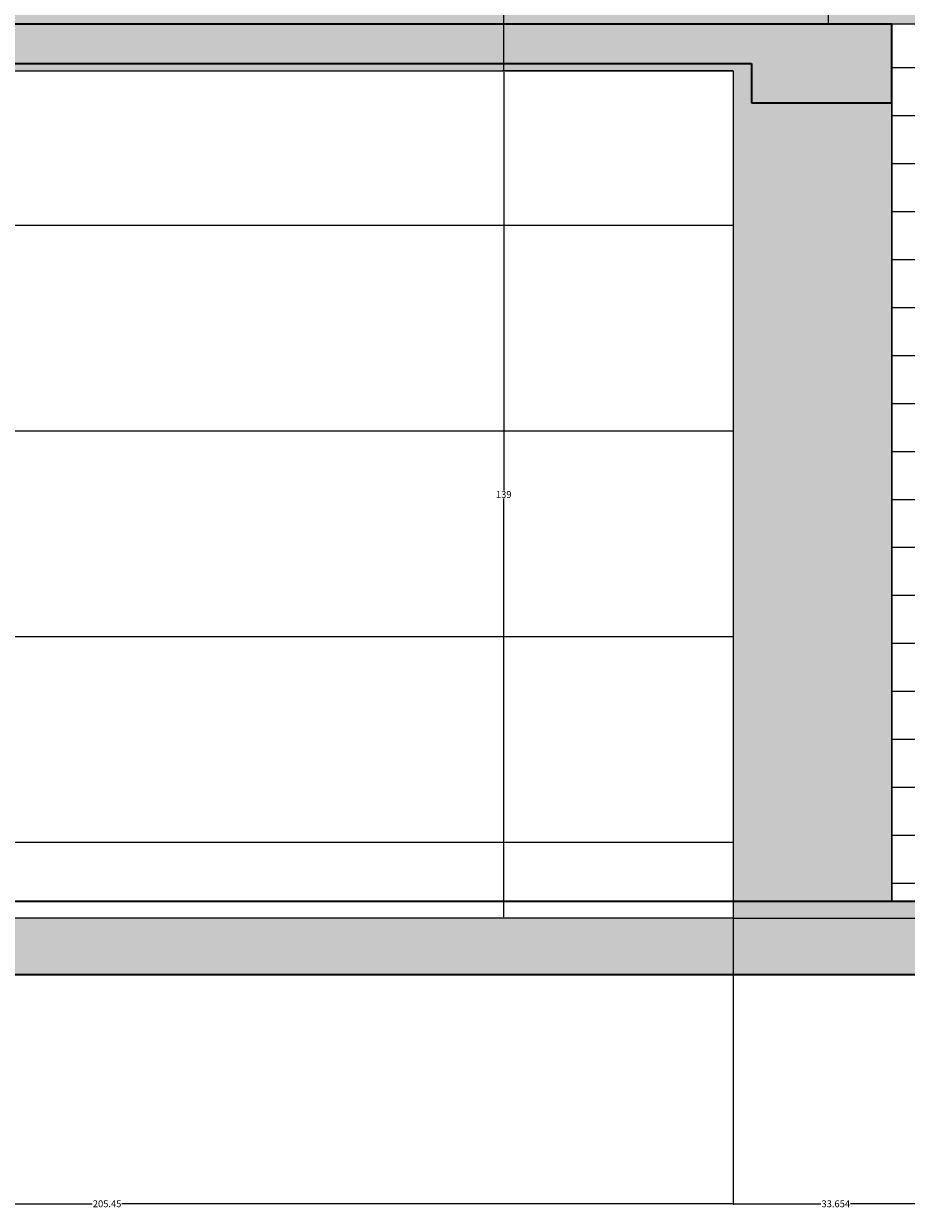
# Model space of a CAD drawing. Units: inches. Extents: x 8 to 634, y 41 to 867.
# Tile 2 of 21: x 153 to 297, y 41 to 236. Entities that reach past the tile are written whole.
import ezdxf

# ---------------------------------------------------------------- set-up
doc = ezdxf.new("R2010")
doc.units = ezdxf.units.IN
doc.header["$MEASUREMENT"] = 0
for name, color, linetype, lineweight in [('A-ANNO-DIMS', 2, 'Continuous', 18), ('A-DOOR', 3, 'Continuous', 25), ('A-DOOR-PATT', 8, 'Continuous', 9), ('A-FLOR', 7, 'Continuous', 35), ('A-FLOR-PATT', 8, 'Continuous', 9), ('A-WALL', 7, 'Continuous', 35), ('A-WALL-PANL', 7, 'Continuous', 18), ('A-WALL-PATT', 8, 'Continuous', 9)]:
    doc.layers.add(name, color=color, linetype=linetype, lineweight=lineweight)
doc.styles.get("Standard").update_dxf_attribs({"font": 'arial.ttf'})
doc.dimstyles.get("Standard").update_dxf_attribs({"dimtxt": 1.125, "dimasz": 0.18, "dimexe": 0.18, "dimexo": 0.0625, "dimgap": 0.09, "dimtad": 0, "dimtih": 1, "dimtoh": 1, "dimdec": 4, "dimzin": 0, "dimdsep": 46, "dimlunit": 4, "dimtxsty": 'Standard', "dimcen": 0.09, "dimadec": 0, "dimazin": 0, "dimtfac": 1, "dimtdec": 4, "dimtofl": 0, "dimtmove": 0, "dimatfit": 3, "dimfxl": 1, "dimtolj": 1, "dimtzin": 0, "dimarcsym": 0})

# ---------------------------------------------------------------- blocks, each defined once
blk = doc.blocks.new('*D29')
at = {"layer": 'A-ANNO-DIMS', "color": 0, "lineweight": -2, "transparency": 16777216}
for p, q in [((63.54, 88.73), (63.54, 41.73)), ((269, 88.73), (269, 41.73)), ((63.72, 41.91), (163.83, 41.91)), ((268.82, 41.91), (168.71, 41.91))]:
    blk.add_line(p, q, dxfattribs=at)
at = {"layer": 'A-ANNO-DIMS', "color": 0, "transparency": 16777216}
for points in [[(63.72, 41.94), (63.72, 41.88), (63.54, 41.91)], [(268.82, 41.94), (268.82, 41.88), (269, 41.91)]]:
    blk.add_solid(points, dxfattribs=at)
at = {"layer": 'Defpoints', "color": 0, "transparency": 16777216}
for p in [(63.54, 88.79), (269, 88.79), (269, 41.91)]:
    blk.add_point(p, dxfattribs=at)
at = {"layer": 'A-ANNO-DIMS', "color": 0, "transparency": 16777216, "insert": (166.27, 41.91), "char_height": 1.125, "attachment_point": 5}
blk.add_mtext('\\A1;205.45', dxfattribs=at)
blk = doc.blocks.new('*D30')
at = {"layer": 'A-ANNO-DIMS', "color": 0, "lineweight": -2, "transparency": 16777216}
for p, q in [((302.65, 100.94), (302.65, 41.73)), ((269, 88.73), (269, 41.73)), ((269.18, 41.91), (283.4, 41.91)), ((302.47, 41.91), (288.25, 41.91))]:
    blk.add_line(p, q, dxfattribs=at)
at = {"layer": 'A-ANNO-DIMS', "color": 0, "transparency": 16777216}
for points in [[(269.18, 41.94), (269.18, 41.88), (269, 41.91)], [(302.47, 41.94), (302.47, 41.88), (302.65, 41.91)]]:
    blk.add_solid(points, dxfattribs=at)
at = {"layer": 'Defpoints', "color": 0, "transparency": 16777216}
for p in [(302.65, 101), (269, 88.79), (302.65, 41.91)]:
    blk.add_point(p, dxfattribs=at)
at = {"layer": 'A-ANNO-DIMS', "color": 0, "transparency": 16777216, "insert": (285.83, 41.91), "char_height": 1.125, "attachment_point": 5}
blk.add_mtext('\\A1;33.654', dxfattribs=at)
blk = doc.blocks.new('*D34')
at = {"layer": 'A-ANNO-DIMS', "color": 0, "lineweight": -2, "transparency": 16777216}
for p, q in [((268.94, 227.8), (231.17, 227.8)), ((231.35, 227.62), (231.35, 158.96)), ((231.35, 88.97), (231.35, 157.63)), ((268.94, 88.79), (231.17, 88.79))]:
    blk.add_line(p, q, dxfattribs=at)
at = {"layer": 'A-ANNO-DIMS', "color": 0, "transparency": 16777216}
for points in [[(231.32, 227.62), (231.38, 227.62), (231.35, 227.8)], [(231.32, 88.97), (231.38, 88.97), (231.35, 88.79)]]:
    blk.add_solid(points, dxfattribs=at)
at = {"layer": 'Defpoints', "color": 0, "transparency": 16777216}
for p in [(231.35, 227.8), (269, 227.8), (269, 88.79)]:
    blk.add_point(p, dxfattribs=at)
at = {"layer": 'A-ANNO-DIMS', "color": 0, "transparency": 16777216, "insert": (231.35, 158.3), "char_height": 1.125, "attachment_point": 5}
blk.add_mtext('\\A1;139', dxfattribs=at)
blk = doc.blocks.new('*D36')
at = {"layer": 'A-ANNO-DIMS', "color": 0, "lineweight": -2, "transparency": 16777216}
for p, q in [((269.06, 88.79), (632.18, 88.79)), ((632, 88.61), (632, 84.84)), ((632, 79.74), (632, 83.51)), ((594.41, 79.56), (632.18, 79.56))]:
    blk.add_line(p, q, dxfattribs=at)
at = {"layer": 'A-ANNO-DIMS', "color": 0, "transparency": 16777216}
for points in [[(631.97, 88.61), (632.03, 88.61), (632, 88.79)], [(631.97, 79.74), (632.03, 79.74), (632, 79.56)]]:
    blk.add_solid(points, dxfattribs=at)
at = {"layer": 'Defpoints', "color": 0, "transparency": 16777216}
for p in [(269, 88.79), (632, 88.79), (594.35, 79.56)]:
    blk.add_point(p, dxfattribs=at)
at = {"layer": 'A-ANNO-DIMS', "color": 0, "transparency": 16777216, "insert": (632, 84.17), "char_height": 1.125, "attachment_point": 5}
blk.add_mtext('\\A1;9.236', dxfattribs=at)
blk = doc.blocks.new('*D37')
at = {"layer": 'A-ANNO-DIMS', "color": 0, "lineweight": -2, "transparency": 16777216}
for p, q in [((353.52, 101), (632.18, 101)), ((632, 100.82), (632, 95.55)), ((632, 88.97), (632, 94.24)), ((269.06, 88.79), (632.18, 88.79))]:
    blk.add_line(p, q, dxfattribs=at)
at = {"layer": 'A-ANNO-DIMS', "color": 0, "transparency": 16777216}
for points in [[(631.97, 100.82), (632.03, 100.82), (632, 101)], [(631.97, 88.97), (632.03, 88.97), (632, 88.79)]]:
    blk.add_solid(points, dxfattribs=at)
at = {"layer": 'Defpoints', "color": 0, "transparency": 16777216}
for p in [(353.46, 101), (632, 101), (269, 88.79)]:
    blk.add_point(p, dxfattribs=at)
at = {"layer": 'A-ANNO-DIMS', "color": 0, "transparency": 16777216, "insert": (632, 94.9), "char_height": 1.125, "attachment_point": 5}
blk.add_mtext('\\A1;12.21', dxfattribs=at)
blk = doc.blocks.new('*D42')
at = {"layer": 'A-ANNO-DIMS', "color": 0, "lineweight": -2, "transparency": 16777216}
for p, q in [((268.93, 284.24), (231.16, 284.23)), ((231.34, 284.05), (231.34, 256.68)), ((231.35, 227.98), (231.34, 255.35)), ((268.94, 227.8), (231.17, 227.8))]:
    blk.add_line(p, q, dxfattribs=at)
at = {"layer": 'A-ANNO-DIMS', "color": 0, "transparency": 16777216}
for points in [[(231.37, 284.05), (231.31, 284.05), (231.34, 284.23)], [(231.38, 227.98), (231.32, 227.98), (231.35, 227.8)]]:
    blk.add_solid(points, dxfattribs=at)
at = {"layer": 'Defpoints', "color": 0, "transparency": 16777216}
for p in [(231.34, 284.23), (268.99, 284.24), (269, 227.8)]:
    blk.add_point(p, dxfattribs=at)
at = {"layer": 'A-ANNO-DIMS', "color": 0, "transparency": 16777216, "insert": (231.34, 256.02), "char_height": 1.125, "attachment_point": 5}
blk.add_mtext('\\A1;56.44', dxfattribs=at)

msp = doc.modelspace()

# ---------------------------------------------------------------- hatches: boundary and pattern name
at = {"layer": 'A-DOOR-PATT', "transparency": 33554687}
h = msp.add_hatch(dxfattribs=at)
h.set_pattern_fill('ANSI31', color=256, scale=270, angle=135)
h.paths.add_polyline_path([(268.998, 227.8036), (63.5448, 227.8036), (63.5448, 91.5555), (268.998, 91.5555)])
at = {"layer": 'A-FLOR-PATT', "transparency": 33554687}
h = msp.add_hatch(dxfattribs=at)
h.set_pattern_fill('AR-CONC', color=256, scale=0.76, angle=135)
h.set_pattern_definition([(185, (0, 0), (-3.517334, 4.191795), [0.57, -6.27]), (130, (0, 0), (-3.29664, -4.78794), [0.456, -5.016]), (235.4514, (-0.293, 0.3493), (-6.81397, -0.596145), [0.484425, -5.32868]), (181.1842, (-1.075, -1.075), (-4.845865, 6.62487), [0.855, -9.405]), (231.6356, (-1.479, -0.523), (-10.25781, -0.21204), [0.72664, -7.99302]), (126.1842, (-1.075, -1.075), (-10.25781, -0.21204), [0.684, -7.524]), (156, (-1.3435, -0.2687), (-1.044107, 5.371464), [0.57, -6.27]), (101, (-1.3435, -0.2687), (-5.204544, -2.589385), [0.456, -5.016]), (206.4514, (-1.4305, 0.179), (-6.24865, 2.78208), [0.484425, -5.32868]), (172.5, (0, 0), (-1.8543226, -1.723628), [0, -4.9552, 0, -5.092, 0, -5.035]), (142.5, (0, 0), (-3.533312, -0.705834), [0, -2.9032, 0, -4.8412, 0, -1.919]), (102.5, (1.1984, -1.1984), (-2.747558, 2.989978), [0, -1.9, 0, -5.928, 0, -7.866]), (92.5, (1.7358, -1.7358), (-3.672015, 2.596084), [0, -2.47, 0, -3.9368, 0, -5.586])])
h.paths.add_polyline_path([(594.3501, 91.5417), (360.785, 91.5417), (295.0049, 91.5417), (268.998, 91.5432), (268.998, 88.7912), (63.5448, 88.7912), (63.5448, 91.5555), (47.3401, 91.5555), (47.3401, 79.5555), (349.489, 79.5555), (594.3501, 79.5555)])
at = {"layer": 'A-WALL-PATT', "transparency": 33554687}
h = msp.add_hatch(dxfattribs=at)
h.set_pattern_fill('AR-CONC', color=256, scale=3.2)
h.paths.add_polyline_path([(119.7065, 697.6655), (47.3401, 697.6655), (47.3401, 569.1705), (119.7065, 569.1705)])
h.paths.add_polyline_path([(202.1558, 697.6655), (119.7065, 697.6655), (119.7065, 569.1705), (202.1558, 569.1705)])
h.paths.add_polyline_path([(284.6051, 697.6655), (202.1558, 697.6655), (202.1558, 569.1705), (284.6051, 569.1705)])
h.paths.add_polyline_path([(119.7065, 569.1705), (47.3401, 569.1705), (47.3401, 523.5555), (47.3401, 449.7533), (119.7065, 449.7533)])
h.paths.add_polyline_path([(342.6544, 682.1444), (360.785, 697.6655), (284.6051, 697.6655), (284.6051, 569.1705), (342.6544, 569.1705)])
h.paths.add_polyline_path([(342.6544, 569.1705), (284.6051, 569.1705), (284.6051, 449.7533), (342.6544, 449.7533)])
h.paths.add_polyline_path([(418.2881, 691.978), (418.2881, 697.6655), (360.785, 697.6655), (360.785, 569.1705), (418.2881, 569.1705)])
h.paths.add_polyline_path([(418.2881, 569.1705), (360.785, 569.1705), (360.785, 523.5555), (360.785, 449.7533), (418.2881, 449.7533)])
h.paths.add_polyline_path([(594.3501, 697.6655), (539.0002, 697.6655), (539.0002, 691.978), (539.0002, 569.1705), (594.3501, 569.1705)])
h.paths.add_polyline_path([(594.3501, 523.5555), (594.3501, 569.1705), (539.0002, 569.1705), (539.0002, 451.6305), (594.3501, 451.6305)])
h.paths.add_polyline_path([(594.3501, 451.6305), (539.0002, 451.6305), (539.0002, 391.7598), (594.3501, 391.7598)])
h.paths.add_polyline_path([(594.3501, 391.7598), (539.0002, 391.7598), (539.0002, 276.166), (594.3501, 276.166)])
h.paths.add_polyline_path([(418.2881, 449.7533), (360.785, 449.7533), (360.785, 391.7598), (418.2881, 391.7598)])
h.paths.add_polyline_path([(342.6544, 449.7533), (284.6051, 449.7533), (284.6051, 391.7598), (342.6544, 391.7598)])
h.paths.add_polyline_path([(342.6544, 391.7598), (284.6051, 391.7598), (284.6051, 272.3426), (342.6544, 272.3426)])
h.paths.add_polyline_path([(418.2881, 391.7598), (360.785, 391.7598), (360.785, 272.3426), (418.2881, 272.3426)])
h.paths.add_polyline_path([(418.2881, 272.3426), (360.785, 272.3426), (360.785, 235.5555), (418.2881, 235.5555)])
h.paths.add_polyline_path([(342.6544, 272.3426), (284.6051, 272.3426), (284.6051, 235.5555), (295.0049, 235.5555), (342.6544, 235.5555)])
h.paths.add_polyline_path([(594.3501, 276.166), (539.0002, 276.166), (539.0002, 228.4951), (594.3501, 228.4951)])
h.paths.add_polyline_path([(594.3501, 228.4951), (539.0002, 228.4951), (539.0002, 91.5417), (594.3501, 91.5417)])
h.paths.add_polyline_path([(418.2881, 235.5555), (360.785, 235.5555), (360.785, 91.5417), (418.2881, 91.5417)])
h.paths.add_polyline_path([(284.6051, 272.3426), (119.7065, 272.3426), (119.7065, 235.5555), (284.6051, 235.5555)])
h.paths.add_polyline_path([(119.7065, 272.3426), (47.3401, 272.3426), (47.3401, 235.5555), (47.3401, 91.5555), (63.5448, 91.5555), (63.5448, 227.8036), (268.998, 227.8036), (268.998, 91.5555), (295.0049, 91.5555), (295.0049, 222.583), (271.9787, 222.583), (271.9787, 229.0481), (62.4019, 229.0481), (62.4019, 222.583), (61.1827, 222.583), (61.1827, 235.5555), (119.7065, 235.5555)])
h.paths.add_polyline_path([(119.7065, 391.7598), (47.3401, 391.7598), (47.3401, 379.5555), (47.3401, 272.3426), (119.7065, 272.3426)])
h.paths.add_polyline_path([(119.7065, 449.7533), (47.3401, 449.7533), (47.3401, 391.7598), (119.7065, 391.7598)])
h.paths.add_polyline_path([(202.1558, 449.7533), (119.7065, 449.7533), (119.7065, 391.7598), (202.1558, 391.7598)])
h.paths.add_polyline_path([(284.6051, 449.7533), (202.1558, 449.7533), (202.1558, 391.7598), (284.6051, 391.7598)])
at = {"layer": 'A-WALL-PATT', "transparency": 33554681}
h = msp.add_hatch(dxfattribs=at)
h.set_pattern_fill('ANSI31', color=256, scale=63, angle=135)
h.paths.add_polyline_path([(284.6051, 391.7598), (119.7065, 391.7598), (119.7065, 272.3426), (284.6051, 272.3426)])
h.paths.add_polyline_path([(193.1116, 284.2398), (131.8771, 284.2398), (131.8771, 380.0085), (193.1116, 380.0085)], flags=16)
h.paths.add_polyline_path([(207.7547, 380.0085), (268.9893, 380.0085), (268.9893, 284.2398), (207.7547, 284.2398)], flags=16)
h.paths.add_polyline_path([(342.6544, 235.5555), (295.0049, 235.5555), (295.0049, 91.5417), (342.6544, 91.5417)])
at = {"layer": 'A-WALL-PATT', "transparency": 33554554}
h = msp.add_hatch(dxfattribs=at)
h.set_pattern_fill('AR-CONC', color=256, scale=0.76, angle=135)
h.paths.add_polyline_path([(295.0049, 235.5555), (61.1827, 235.5555), (61.1827, 222.583), (62.4019, 222.583), (62.4019, 229.0481), (271.9787, 229.0481), (271.9787, 222.583), (295.0049, 222.583)])

# ---------------------------------------------------------------- linework, layer by layer
at = {"layer": 'A-DOOR'}
msp.add_line((295.0049, 222.583), (295.0049, 91.5555), dxfattribs=at)
for points in [[(295.0049, 235.5555), (360.785, 235.5555), (360.785, 91.5417), (295.0049, 91.5417)], [(63.5448, 227.8036), (268.998, 227.8036), (268.998, 88.7912), (63.5448, 88.7912)]]:
    msp.add_lwpolyline(points, close=True, dxfattribs=at)
at = {"layer": 'A-FLOR'}
for p, q in [((47.3401, 91.5555), (349.489, 91.5555)), ((47.3401, 79.5555), (349.489, 79.5555))]:
    msp.add_line(p, q, dxfattribs=at)
at = {"layer": 'A-WALL'}
for p, q in [((61.1827, 235.5555), (295.0049, 235.5555)), ((295.0049, 222.583), (295.0049, 235.5555)), ((62.4019, 229.0481), (271.9787, 229.0481)), ((271.9787, 229.0481), (271.9787, 222.583)), ((271.9787, 222.583), (295.0049, 222.583))]:
    msp.add_line(p, q, dxfattribs=at)
at = {"layer": 'A-WALL-PANL'}
msp.add_line((284.6051, 272.3426), (284.6051, 235.5555), dxfattribs=at)

# ---------------------------------------------------------------- dimensions: what is measured, and where the dimension line sits
at = {"layer": 'A-ANNO-DIMS'}
for base, p1, p2, angle, override, picture, middle in [((231.3393, 284.234), (268.998, 227.8036), (268.9893, 284.2398), 90.00885, {"dimdec": 2, "dimlfac": 1, "dimrnd": 0, "dimzin": 0, "dimdsep": 46, "dimlunit": 2}, '*D42', (231.3436, 256.0159)), ((231.348, 227.8036), (268.998, 88.7912), (268.998, 227.8036), 90, {"dimdec": 0, "dimlfac": 1, "dimrnd": 0, "dimzin": 0, "dimdsep": 46, "dimlunit": 2}, '*D34', (231.348, 158.2974)), ((632.0001, 101.0012), (268.998, 88.7912), (353.4573, 101.0012), 90, {"dimdec": 2, "dimlfac": 1, "dimrnd": 0, "dimzin": 0, "dimdsep": 46, "dimlunit": 2}, '*D37', (632.0001, 94.8962)), ((632.0001, 88.7912), (594.3501, 79.5555), (268.998, 88.7912), 90, {"dimdec": 3, "dimlfac": 1, "dimrnd": 0, "dimzin": 0, "dimdsep": 46, "dimlunit": 2}, '*D36', (632.0001, 84.1734))]:
    dim = msp.add_linear_dim(base=base, p1=p1, p2=p2, angle=angle, dimstyle='Standard', override=override, dxfattribs=at)
    dim.commit()
    dim.dimension.update_dxf_attribs({"geometry": picture, "text_midpoint": middle})
for base, p1, p2, override, picture, middle in [((302.6522, 41.9055), (268.998, 88.7912), (302.6522, 101.0012), {"dimdec": 3, "dimlfac": 1, "dimrnd": 0, "dimzin": 0, "dimdsep": 46, "dimlunit": 2}, '*D30', (285.8251, 41.9055)), ((268.998, 41.9055), (63.5448, 88.7912), (268.998, 88.7912), {"dimdec": 2, "dimlfac": 1, "dimrnd": 0, "dimzin": 0, "dimdsep": 46, "dimlunit": 2}, '*D29', (166.2714, 41.9055))]:
    dim = msp.add_linear_dim(base=base, p1=p1, p2=p2, dimstyle='Standard', override=override, dxfattribs=at)
    dim.commit()
    dim.dimension.update_dxf_attribs({"geometry": picture, "text_midpoint": middle})

doc.saveas('drawing.dxf')
